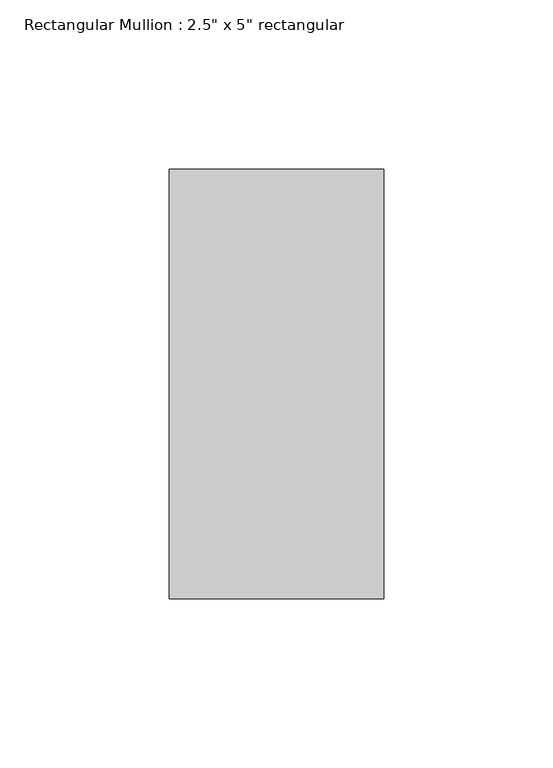
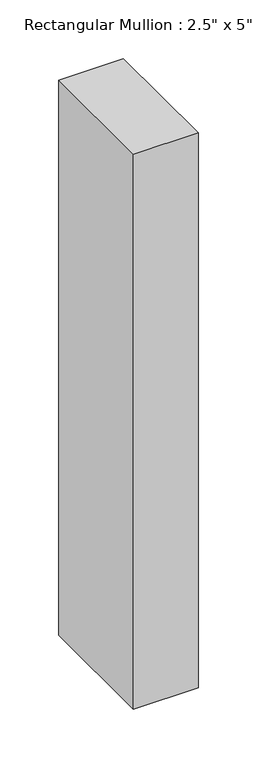
"""IFC4 building model written with IfcOpenShell, lengths in millimetres: member geometry."""

from ifc_helpers import new_model, si_unit, frame, origin, place, context, project, spatial, polyline, outline, extrude, source, transform, mapped, element, save


def member_504574e5(model_context):
    return source(origin(), model_context, "Body", "SweptSolid", [
        extrude(outline(polyline([(0.0, 63.5), (0.0, -63.5), (-63.5, -63.5), (-63.5, 63.5), (0.0, 63.5)])), frame((0.0, 0.0, -575.8872143), z_axis=(0.0, 0.0, 1.0), x_axis=(1.0, 0.0, 0.0)), (0.0, 0.0, 1.0), 575.8872143),
    ])


if __name__ == "__main__":
    model = new_model("IFC4")
    model_context = context("Model", 3, world=origin())
    ifc_project = project(units=[si_unit("LENGTHUNIT", "METRE", prefix="MILLI")], contexts=[model_context])
    site = spatial("IfcSite", under=ifc_project)
    building = spatial("IfcBuilding", under=site)
    placement = place(None, origin())
    member_shape = member_504574e5(model_context)
    element("IfcMember", 1, ObjectType="Rectangular Mullion : 2.5\" x 5\" rectangular", at=placement, inside=building, context=model_context, shape_type="MappedRepresentation", body=[
        mapped(member_shape, transform((0.0, 0.0, 0.0), x_axis=(1.0, 0.0, 0.0), y_axis=(0.0, 1.0, 0.0), z_axis=(0.0, 0.0, 1.0))),
    ])
    save(model, "model.ifc")

# Revit data of these elements
# Type "Rectangular Mullion : 2.5\" x 5\" rectangular"
#   built-in parameter 1007304 = 0.416667 (stored number, unit not read)
#   built-in parameter 1007301 = 0.104167 (stored number, unit not read)
#   built-in parameter 1007300 = 0.104167 (stored number, unit not read)
# Element 1 (IfcMember, "Rectangular Mullion : 2.5\" x 5\" rectangular")
#   Materials on its faces: "Aluminum"
# Materials
#   "Aluminum": class "Metal", colour RGB 247 247 247, transparency 0, Description = "Aluminum 6061", Cost = 0
